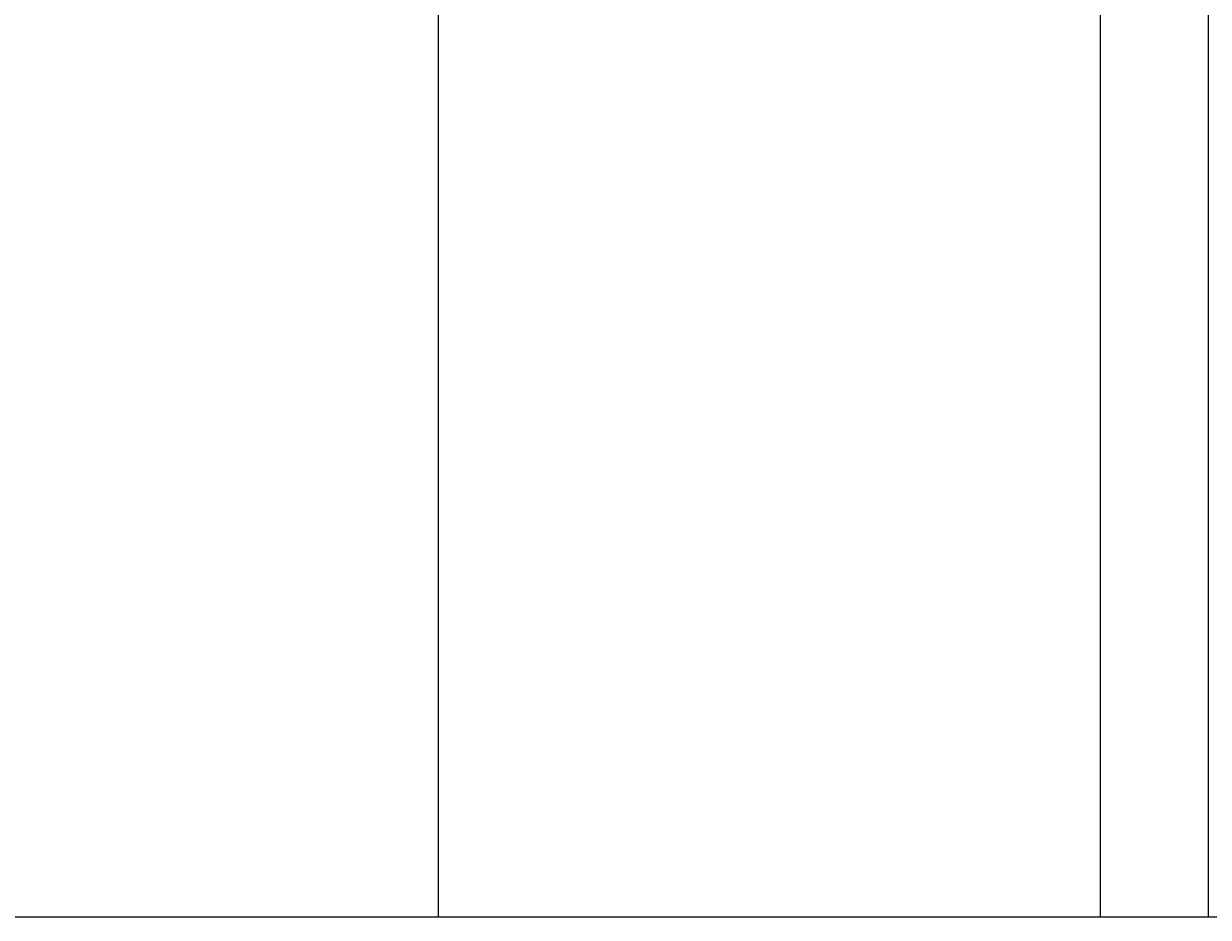
# Model space of a CAD drawing. Units: inches. Extents: x 35362 to 73946, y 43607 to 67532.
# Tile 133 of 134: x 66704 to 68484, y 43607 to 44948. Entities that reach past the tile are written whole.
import ezdxf

# ---------------------------------------------------------------- set-up
doc = ezdxf.new("R2010")
doc.units = ezdxf.units.IN
doc.header["$MEASUREMENT"] = 0
doc.layers.add('A-ANNO-DIMS', color=2, linetype='Continuous', lineweight=18)
doc.styles.get("Standard").update_dxf_attribs({"font": 'arial.ttf'})
doc.dimstyles.get("Standard").update_dxf_attribs({"dimtxt": 0.18, "dimasz": 0.18, "dimexe": 0.18, "dimexo": 0.0625, "dimgap": 0.09, "dimtad": 0, "dimtih": 1, "dimtoh": 1, "dimdec": 4, "dimzin": 0, "dimdsep": 46, "dimtxsty": 'Standard', "dimcen": 0.09, "dimadec": 0, "dimazin": 0, "dimtfac": 1, "dimtdec": 4, "dimtofl": 0, "dimtmove": 0, "dimatfit": 3, "dimfxl": 1, "dimtolj": 1, "dimtzin": 0, "dimarcsym": 0})

# ---------------------------------------------------------------- blocks, each defined once
blk = doc.blocks.new('*D5')
at = {"layer": 'A-ANNO-DIMS', "color": 0, "lineweight": -2, "transparency": 16777216}
for p, q in [((37121.949085, 46919.318283), (37121.949085, 43606.678996)), ((69871.496302, 45449.831951), (69871.496302, 43606.678996)), ((37122.129085, 43606.858996), (53496.2943647142, 43606.858996)), ((69871.316302, 43606.858996), (53497.15102228581, 43606.858996))]:
    blk.add_line(p, q, dxfattribs=at)
at = {"layer": 'A-ANNO-DIMS', "color": 0, "transparency": 16777216}
for points in [[(37122.129085, 43606.888996), (37122.129085, 43606.828996), (37121.949085, 43606.858996)], [(69871.316302, 43606.888996), (69871.316302, 43606.828996), (69871.496302, 43606.858996)]]:
    blk.add_solid(points, dxfattribs=at)
at = {"layer": 'Defpoints', "color": 0, "transparency": 16777216}
for p in [(37121.949085, 46919.380783), (69871.496302, 45449.894451), (69871.496302, 43606.858996)]:
    blk.add_point(p, dxfattribs=at)
at = {"layer": 'A-ANNO-DIMS', "color": 0, "transparency": 16777216, "insert": (53496.7226935, 43606.858996), "char_height": 0.18, "attachment_point": 5}
blk.add_mtext('\\A1;32750', dxfattribs=at)
blk = doc.blocks.new('*D38')
at = {"layer": 'A-ANNO-DIMS', "color": 0, "lineweight": -2, "transparency": 16777216}
for p, q in [((68483.500128, 45449.831951), (68483.500128, 43606.678996)), ((62090.58505699999, 45366.796496), (62090.58505699999, 43606.678996)), ((62090.76505699999, 43606.858996), (65286.57828827081, 43606.858996)), ((68483.320128, 43606.858996), (65287.5068967292, 43606.858996))]:
    blk.add_line(p, q, dxfattribs=at)
at = {"layer": 'A-ANNO-DIMS', "color": 0, "transparency": 16777216}
for points in [[(62090.76505699999, 43606.888996), (62090.76505699999, 43606.828996), (62090.58505699999, 43606.858996)], [(68483.320128, 43606.888996), (68483.320128, 43606.828996), (68483.500128, 43606.858996)]]:
    blk.add_solid(points, dxfattribs=at)
at = {"layer": 'Defpoints', "color": 0, "transparency": 16777216}
for p in [(68483.500128, 45449.894451), (62090.58505699999, 45366.858996), (68483.500128, 43606.858996)]:
    blk.add_point(p, dxfattribs=at)
at = {"layer": 'A-ANNO-DIMS', "color": 0, "transparency": 16777216, "insert": (65287.0425925, 43606.858996), "char_height": 0.18, "attachment_point": 5}
blk.add_mtext('\\A1;6392.9', dxfattribs=at)
blk = doc.blocks.new('*D65')
at = {"layer": 'A-ANNO-DIMS', "color": 0, "lineweight": -2, "transparency": 16777216}
for p, q in [((65336.01600799999, 61293.223552), (65336.01600799999, 43606.678996)), ((67326.639741, 61293.223552), (67326.639741, 43606.678996)), ((65336.19600799999, 43606.858996), (66330.87277900206, 43606.858996)), ((67326.45974100001, 43606.858996), (66331.78296999796, 43606.858996))]:
    blk.add_line(p, q, dxfattribs=at)
at = {"layer": 'A-ANNO-DIMS', "color": 0, "transparency": 16777216}
for points in [[(65336.19600799999, 43606.888996), (65336.19600799999, 43606.828996), (65336.01600799999, 43606.858996)], [(67326.45974100001, 43606.888996), (67326.45974100001, 43606.828996), (67326.639741, 43606.858996)]]:
    blk.add_solid(points, dxfattribs=at)
at = {"layer": 'Defpoints', "color": 0, "transparency": 16777216}
for p in [(65336.01600799999, 61293.286052), (67326.639741, 61293.286052), (67326.639741, 43606.858996)]:
    blk.add_point(p, dxfattribs=at)
at = {"layer": 'A-ANNO-DIMS', "color": 0, "transparency": 16777216, "insert": (66331.32787450001, 43606.858996), "char_height": 0.18, "attachment_point": 5}
blk.add_mtext('\\A1;1990.6', dxfattribs=at)
blk = doc.blocks.new('*D68')
at = {"layer": 'A-ANNO-DIMS', "color": 0, "lineweight": -2, "transparency": 16777216}
for p, q in [((68320.870762, 54372.885224), (68320.870762, 43606.678996)), ((61240.907336, 53351.466162), (61240.907336, 43606.678996)), ((61241.08733599999, 43606.858996), (64780.42646373397, 43606.858996)), ((68320.69076200001, 43606.858996), (64781.35163426603, 43606.858996))]:
    blk.add_line(p, q, dxfattribs=at)
at = {"layer": 'A-ANNO-DIMS', "color": 0, "transparency": 16777216}
for points in [[(61241.08733599999, 43606.888996), (61241.08733599999, 43606.828996), (61240.907336, 43606.858996)], [(68320.69076200001, 43606.888996), (68320.69076200001, 43606.828996), (68320.870762, 43606.858996)]]:
    blk.add_solid(points, dxfattribs=at)
at = {"layer": 'Defpoints', "color": 0, "transparency": 16777216}
for p in [(68320.870762, 54372.947724), (61240.907336, 53351.52866199999), (68320.870762, 43606.858996)]:
    blk.add_point(p, dxfattribs=at)
at = {"layer": 'A-ANNO-DIMS', "color": 0, "transparency": 16777216, "insert": (64780.889049, 43606.858996), "char_height": 0.18, "attachment_point": 5}
blk.add_mtext('\\A1;7080.0', dxfattribs=at)

msp = doc.modelspace()

# ---------------------------------------------------------------- dimensions: what is measured, and where the dimension line sits
at = {"layer": 'A-ANNO-DIMS'}
for base, p1, p2, override, picture, middle in [((67326.639741, 43606.858996), (65336.01600799999, 61293.286052), (67326.639741, 61293.286052), {"dimdec": 1, "dimlfac": 1, "dimrnd": 0, "dimzin": 0, "dimdsep": 46, "dimlunit": 2}, '*D65', (66331.32787450001, 43606.858996)), ((68320.870762, 43606.858996), (61240.907336, 53351.52866199999), (68320.870762, 54372.947724), {"dimdec": 1, "dimlfac": 1, "dimrnd": 0, "dimzin": 0, "dimdsep": 46, "dimlunit": 2}, '*D68', (64780.889049, 43606.858996)), ((69871.496302, 43606.858996), (37121.949085, 46919.380783), (69871.496302, 45449.894451), {"dimdec": 0, "dimlfac": 1, "dimrnd": 0, "dimzin": 0, "dimdsep": 46, "dimlunit": 2}, '*D5', (53496.7226935, 43606.858996)), ((68483.500128, 43606.858996), (62090.58505699999, 45366.858996), (68483.500128, 45449.894451), {"dimdec": 1, "dimlfac": 1, "dimrnd": 0, "dimzin": 0, "dimdsep": 46, "dimlunit": 2}, '*D38', (65287.0425925, 43606.858996))]:
    dim = msp.add_linear_dim(base=base, p1=p1, p2=p2, dimstyle='Standard', override=override, dxfattribs=at)
    dim.commit()
    dim.dimension.update_dxf_attribs({"geometry": picture, "text_midpoint": middle})

doc.saveas('drawing.dxf')
